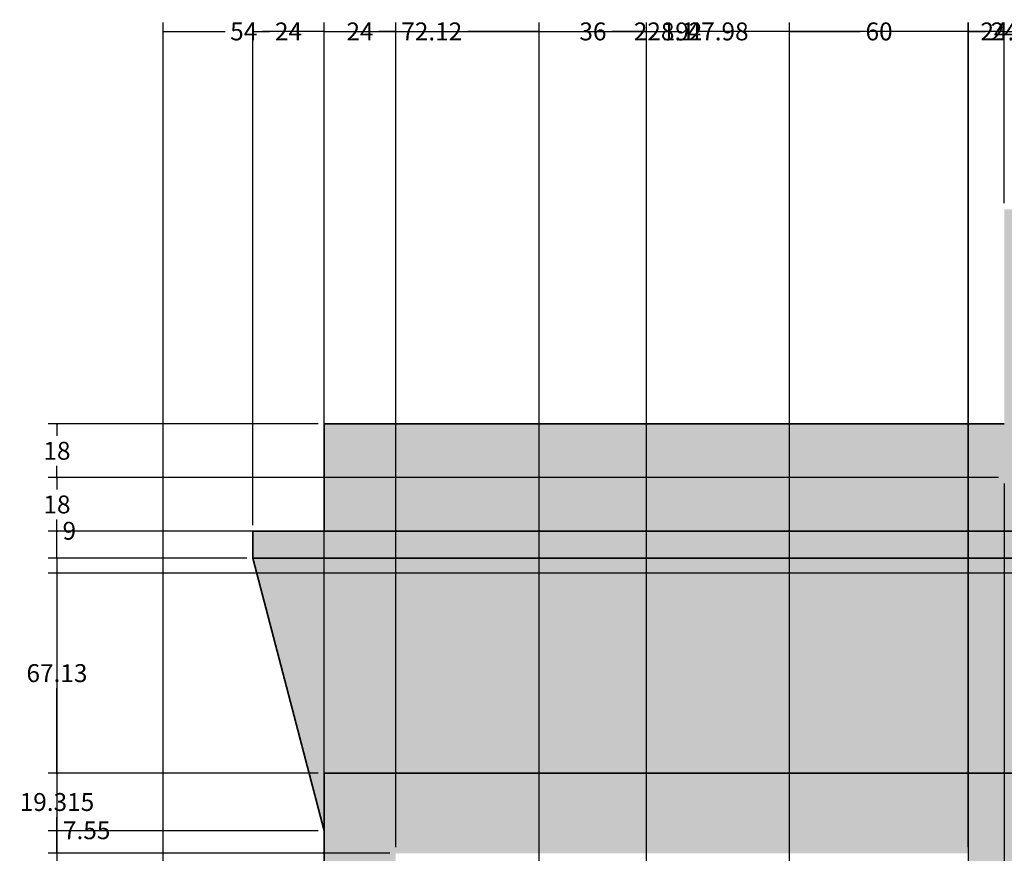
# Model space of a CAD drawing. Units: inches. Extents: x 860 to 1491, y 583 to 1370.
# Tile 7 of 8: x 860 to 1190, y 1091 to 1370. Entities that reach past the tile are written whole.
import ezdxf

# ---------------------------------------------------------------- set-up
doc = ezdxf.new("R2010")
doc.units = ezdxf.units.IN
doc.header["$MEASUREMENT"] = 0
doc.layers.get('0').update_dxf_attribs({"color": 250})
for name, color, linetype, lineweight in [('A-ANNO-DIMS', 2, 'Continuous', 18), ('A-ELEV', 7, 'Continuous', 35), ('A-ELEV-PATT', 9, 'Continuous', 13)]:
    doc.layers.add(name, color=color, linetype=linetype, lineweight=lineweight)
doc.styles.get("Standard").update_dxf_attribs({"font": 'arial.ttf'})
doc.dimstyles.get("Standard").update_dxf_attribs({"dimtxt": 6, "dimasz": 0.18, "dimexe": 3, "dimexo": 2, "dimgap": 2, "dimtad": 0, "dimtih": 1, "dimtoh": 1, "dimdec": 0, "dimzin": 0, "dimdsep": 46, "dimlunit": 3, "dimtxsty": 'Standard', "dimblk2": 'CLOSEDBLANK', "dimsah": 1, "dimcen": 2, "dimadec": 0, "dimazin": 0, "dimtfac": 1, "dimtdec": 0, "dimtofl": 0, "dimtmove": 0, "dimatfit": 3, "dimfxl": 1, "dimtolj": 1, "dimtzin": 0, "dimarcsym": 0})

# ---------------------------------------------------------------- blocks, each defined once
blk = doc.blocks.new('_ClosedBlank')
at = {"color": 0, "linetype": 'ByBlock', "lineweight": -2}
for p, q in [((-1, 0.17), (0, 0)), ((-1, 0.17), (-1, -0.17)), ((0, 0), (-1, -0.17))]:
    blk.add_line(p, q, dxfattribs=at)
blk = doc.blocks.new('*D2')
at = {"layer": 'A-ANNO-DIMS', "color": 0, "lineweight": -2, "transparency": 16777216}
for p, q in [((1442.44, 1328.76), (1442.44, 584.11)), ((908.34, 740.76), (908.34, 584.11)), ((908.52, 587.11), (1163.85, 587.11)), ((1442.26, 587.11), (1186.93, 587.11))]:
    blk.add_line(p, q, dxfattribs=at)
at = {"layer": 'A-ANNO-DIMS', "color": 0, "transparency": 16777216}
blk.add_solid([(908.52, 587.14), (908.52, 587.08), (908.34, 587.11)], dxfattribs=at)
at = {"layer": 'Defpoints', "color": 0, "transparency": 16777216}
for p in [(1442.44, 1330.76), (908.34, 742.76), (1442.44, 587.11)]:
    blk.add_point(p, dxfattribs=at)
at = {"layer": 'A-ANNO-DIMS', "color": 0, "lineweight": -2, "transparency": 16777216, "xscale": 0.18, "yscale": 0.18, "zscale": 0.18}
blk.add_blockref('_ClosedBlank', (1442.44, 587.11), dxfattribs=at)
at = {"layer": 'A-ANNO-DIMS', "color": 0, "transparency": 16777216, "insert": (1175.39, 587.11), "char_height": 6, "attachment_point": 5}
blk.add_mtext('\\A1;534.1', dxfattribs=at)
blk = doc.blocks.new('*D5')
at = {"layer": 'A-ANNO-DIMS', "color": 0, "lineweight": -2, "transparency": 16777216}
for p, q in [((936.34, 1189.76), (869.69, 1189.76)), ((872.69, 1189.58), (872.69, 1049.32)), ((872.69, 898.94), (872.69, 1039.19)), ((960.34, 898.76), (869.69, 898.76))]:
    blk.add_line(p, q, dxfattribs=at)
at = {"layer": 'A-ANNO-DIMS', "color": 0, "transparency": 16777216}
blk.add_solid([(872.66, 898.94), (872.72, 898.94), (872.69, 898.76)], dxfattribs=at)
at = {"layer": 'Defpoints', "color": 0, "transparency": 16777216}
for p in [(872.69, 1189.76), (938.34, 1189.76), (962.34, 898.76)]:
    blk.add_point(p, dxfattribs=at)
at = {"layer": 'A-ANNO-DIMS', "color": 0, "lineweight": -2, "transparency": 16777216, "xscale": 0.18, "yscale": 0.18, "zscale": 0.18, "rotation": 90}
blk.add_blockref('_ClosedBlank', (872.69, 1189.76), dxfattribs=at)
at = {"layer": 'A-ANNO-DIMS', "color": 0, "transparency": 16777216, "insert": (872.69, 1044.26), "char_height": 6, "attachment_point": 5}
blk.add_mtext('\\A1;291', dxfattribs=at)
blk = doc.blocks.new('*D20')
at = {"layer": 'A-ANNO-DIMS', "color": 0, "lineweight": -2, "transparency": 16777216}
for p, q in [((908.34, 744.76), (908.34, 1369.41)), ((962.34, 732.76), (962.34, 1369.41)), ((908.52, 1366.41), (929.06, 1366.41)), ((962.16, 1366.41), (941.63, 1366.41))]:
    blk.add_line(p, q, dxfattribs=at)
at = {"layer": 'A-ANNO-DIMS', "color": 0, "transparency": 16777216}
blk.add_solid([(908.52, 1366.44), (908.52, 1366.38), (908.34, 1366.41)], dxfattribs=at)
at = {"layer": 'Defpoints', "color": 0, "transparency": 16777216}
for p in [(962.34, 1366.41), (908.34, 742.76), (962.34, 730.76)]:
    blk.add_point(p, dxfattribs=at)
at = {"layer": 'A-ANNO-DIMS', "color": 0, "lineweight": -2, "transparency": 16777216, "xscale": 0.18, "yscale": 0.18, "zscale": 0.18}
blk.add_blockref('_ClosedBlank', (962.34, 1366.41), dxfattribs=at)
at = {"layer": 'A-ANNO-DIMS', "color": 0, "transparency": 16777216, "insert": (935.34, 1366.41), "char_height": 6, "attachment_point": 5}
blk.add_mtext('\\A1;54', dxfattribs=at)
blk = doc.blocks.new('*D21')
at = {"layer": 'A-ANNO-DIMS', "color": 0, "lineweight": -2, "transparency": 16777216}
for p, q in [((962.34, 732.76), (962.34, 1369.41)), ((1034.46, 828.76), (1034.46, 1369.41)), ((962.52, 1366.41), (986.33, 1366.41)), ((1034.28, 1366.41), (1010.47, 1366.41))]:
    blk.add_line(p, q, dxfattribs=at)
at = {"layer": 'A-ANNO-DIMS', "color": 0, "transparency": 16777216}
blk.add_solid([(962.52, 1366.44), (962.52, 1366.38), (962.34, 1366.41)], dxfattribs=at)
at = {"layer": 'Defpoints', "color": 0, "transparency": 16777216}
for p in [(1034.46, 1366.41), (1034.46, 826.76), (962.34, 730.76)]:
    blk.add_point(p, dxfattribs=at)
at = {"layer": 'A-ANNO-DIMS', "color": 0, "lineweight": -2, "transparency": 16777216, "xscale": 0.18, "yscale": 0.18, "zscale": 0.18}
blk.add_blockref('_ClosedBlank', (1034.46, 1366.41), dxfattribs=at)
at = {"layer": 'A-ANNO-DIMS', "color": 0, "transparency": 16777216, "insert": (998.4, 1366.41), "char_height": 6, "attachment_point": 5}
blk.add_mtext('\\A1;72.12', dxfattribs=at)
blk = doc.blocks.new('*D22')
at = {"layer": 'A-ANNO-DIMS', "color": 0, "lineweight": -2, "transparency": 16777216}
for p, q in [((1034.46, 828.76), (1034.46, 1369.41)), ((1070.46, 828.76), (1070.46, 1369.41)), ((1034.64, 1366.41), (1046.17, 1366.41)), ((1070.28, 1366.41), (1058.75, 1366.41))]:
    blk.add_line(p, q, dxfattribs=at)
at = {"layer": 'A-ANNO-DIMS', "color": 0, "transparency": 16777216}
blk.add_solid([(1034.64, 1366.44), (1034.64, 1366.38), (1034.46, 1366.41)], dxfattribs=at)
at = {"layer": 'Defpoints', "color": 0, "transparency": 16777216}
for p in [(1070.46, 1366.41), (1034.46, 826.76), (1070.46, 826.76)]:
    blk.add_point(p, dxfattribs=at)
at = {"layer": 'A-ANNO-DIMS', "color": 0, "lineweight": -2, "transparency": 16777216, "xscale": 0.18, "yscale": 0.18, "zscale": 0.18}
blk.add_blockref('_ClosedBlank', (1070.46, 1366.41), dxfattribs=at)
at = {"layer": 'A-ANNO-DIMS', "color": 0, "transparency": 16777216, "insert": (1052.46, 1366.41), "char_height": 6, "attachment_point": 5}
blk.add_mtext('\\A1;36', dxfattribs=at)
blk = doc.blocks.new('*D23')
at = {"layer": 'A-ANNO-DIMS', "color": 0, "lineweight": -2, "transparency": 16777216}
for p, q in [((1070.46, 828.76), (1070.46, 1369.41)), ((1118.44, 840.76), (1118.44, 1369.41)), ((1070.64, 1366.41), (1082.2, 1366.41)), ((1118.26, 1366.41), (1106.7, 1366.41))]:
    blk.add_line(p, q, dxfattribs=at)
at = {"layer": 'A-ANNO-DIMS', "color": 0, "transparency": 16777216}
blk.add_solid([(1070.64, 1366.44), (1070.64, 1366.38), (1070.46, 1366.41)], dxfattribs=at)
at = {"layer": 'Defpoints', "color": 0, "transparency": 16777216}
for p in [(1118.44, 1366.41), (1118.44, 838.76), (1070.46, 826.76)]:
    blk.add_point(p, dxfattribs=at)
at = {"layer": 'A-ANNO-DIMS', "color": 0, "lineweight": -2, "transparency": 16777216, "xscale": 0.18, "yscale": 0.18, "zscale": 0.18}
blk.add_blockref('_ClosedBlank', (1118.44, 1366.41), dxfattribs=at)
at = {"layer": 'A-ANNO-DIMS', "color": 0, "transparency": 16777216, "insert": (1094.45, 1366.41), "char_height": 6, "attachment_point": 5}
blk.add_mtext('\\A1;47.98', dxfattribs=at)
blk = doc.blocks.new('*D24')
at = {"layer": 'A-ANNO-DIMS', "color": 0, "lineweight": -2, "transparency": 16777216}
for p, q in [((1118.44, 840.76), (1118.44, 1369.41)), ((1178.44, 840.76), (1178.44, 1369.41)), ((1118.62, 1366.41), (1142.14, 1366.41)), ((1178.26, 1366.41), (1154.74, 1366.41))]:
    blk.add_line(p, q, dxfattribs=at)
at = {"layer": 'A-ANNO-DIMS', "color": 0, "transparency": 16777216}
blk.add_solid([(1118.62, 1366.44), (1118.62, 1366.38), (1118.44, 1366.41)], dxfattribs=at)
at = {"layer": 'Defpoints', "color": 0, "transparency": 16777216}
for p in [(1178.44, 1366.41), (1118.44, 838.76), (1178.44, 838.76)]:
    blk.add_point(p, dxfattribs=at)
at = {"layer": 'A-ANNO-DIMS', "color": 0, "lineweight": -2, "transparency": 16777216, "xscale": 0.18, "yscale": 0.18, "zscale": 0.18}
blk.add_blockref('_ClosedBlank', (1178.44, 1366.41), dxfattribs=at)
at = {"layer": 'A-ANNO-DIMS', "color": 0, "transparency": 16777216, "insert": (1148.44, 1366.41), "char_height": 6, "attachment_point": 5}
blk.add_mtext('\\A1;60', dxfattribs=at)
blk = doc.blocks.new('*D25')
at = {"layer": 'A-ANNO-DIMS', "color": 0, "lineweight": -2, "transparency": 16777216}
for p, q in [((1178.44, 840.76), (1178.44, 1369.41)), ((1202.44, 744.76), (1202.44, 1369.41)), ((1178.62, 1366.41), (1184.1, 1366.41)), ((1202.26, 1366.41), (1196.78, 1366.41))]:
    blk.add_line(p, q, dxfattribs=at)
at = {"layer": 'A-ANNO-DIMS', "color": 0, "transparency": 16777216}
blk.add_solid([(1178.62, 1366.44), (1178.62, 1366.38), (1178.44, 1366.41)], dxfattribs=at)
at = {"layer": 'Defpoints', "color": 0, "transparency": 16777216}
for p in [(1202.44, 1366.41), (1178.44, 838.76), (1202.44, 742.76)]:
    blk.add_point(p, dxfattribs=at)
at = {"layer": 'A-ANNO-DIMS', "color": 0, "lineweight": -2, "transparency": 16777216, "xscale": 0.18, "yscale": 0.18, "zscale": 0.18}
blk.add_blockref('_ClosedBlank', (1202.44, 1366.41), dxfattribs=at)
at = {"layer": 'A-ANNO-DIMS', "color": 0, "transparency": 16777216, "insert": (1190.44, 1366.41), "char_height": 6, "attachment_point": 5}
blk.add_mtext('\\A1;24', dxfattribs=at)
blk = doc.blocks.new('*D44')
at = {"layer": 'A-ANNO-DIMS', "color": 0, "lineweight": -2, "transparency": 16777216}
for p, q in [((984.340309, 1090.755507), (869.690309, 1090.755507)), ((872.690309, 1090.935507), (872.690309, 1091.115507)), ((996.340309, 1078.755507), (869.690309, 1078.755507)), ((872.690309, 1078.575507), (872.690309, 1078.395507))]:
    blk.add_line(p, q, dxfattribs=at)
at = {"layer": 'A-ANNO-DIMS', "color": 0, "transparency": 16777216}
blk.add_solid([(872.660309, 1078.575507), (872.720309, 1078.575507), (872.690309, 1078.755507)], dxfattribs=at)
at = {"layer": 'Defpoints', "color": 0, "transparency": 16777216}
for p in [(872.690309, 1090.755507), (986.340309, 1090.755507), (998.340309, 1078.755507)]:
    blk.add_point(p, dxfattribs=at)
at = {"layer": 'A-ANNO-DIMS', "color": 0, "lineweight": -2, "transparency": 16777216, "xscale": 0.18, "yscale": 0.18, "zscale": 0.18, "rotation": 270}
blk.add_blockref('_ClosedBlank', (872.690309, 1090.755507), dxfattribs=at)
at = {"layer": 'A-ANNO-DIMS', "color": 0, "transparency": 16777216, "insert": (872.690309, 1084.755507), "char_height": 6, "attachment_point": 5}
blk.add_mtext('\\A1;12', dxfattribs=at)
blk = doc.blocks.new('*D45')
at = {"layer": 'A-ANNO-DIMS', "color": 0, "lineweight": -2, "transparency": 16777216}
for p, q in [((960.34, 1098.31), (869.69, 1098.31)), ((872.69, 1098.31), (872.69, 1098.49)), ((872.69, 1098.49), (872.87, 1098.49)), ((872.69, 1090.94), (872.69, 1098.13)), ((984.34, 1090.76), (869.69, 1090.76))]:
    blk.add_line(p, q, dxfattribs=at)
at = {"layer": 'A-ANNO-DIMS', "color": 0, "transparency": 16777216}
blk.add_solid([(872.66, 1090.94), (872.72, 1090.94), (872.69, 1090.76)], dxfattribs=at)
at = {"layer": 'Defpoints', "color": 0, "transparency": 16777216}
for p in [(872.69, 1098.31), (962.34, 1098.31), (986.34, 1090.76)]:
    blk.add_point(p, dxfattribs=at)
at = {"layer": 'A-ANNO-DIMS', "color": 0, "lineweight": -2, "transparency": 16777216, "xscale": 0.18, "yscale": 0.18, "zscale": 0.18, "rotation": 90}
blk.add_blockref('_ClosedBlank', (872.69, 1098.31), dxfattribs=at)
at = {"layer": 'A-ANNO-DIMS', "color": 0, "transparency": 16777216, "insert": (882.66, 1098.49), "char_height": 6, "attachment_point": 5}
blk.add_mtext('\\A1;7.55', dxfattribs=at)
blk = doc.blocks.new('*D46')
at = {"layer": 'A-ANNO-DIMS', "color": 0, "lineweight": -2, "transparency": 16777216}
for p, q in [((960.34, 1117.62), (869.69, 1117.62)), ((872.69, 1117.44), (872.69, 1113.03)), ((872.69, 1098.49), (872.69, 1102.9)), ((960.34, 1098.31), (869.69, 1098.31))]:
    blk.add_line(p, q, dxfattribs=at)
at = {"layer": 'A-ANNO-DIMS', "color": 0, "transparency": 16777216}
blk.add_solid([(872.66, 1098.49), (872.72, 1098.49), (872.69, 1098.31)], dxfattribs=at)
at = {"layer": 'Defpoints', "color": 0, "transparency": 16777216}
for p in [(872.69, 1117.62), (962.34, 1117.62), (962.34, 1098.31)]:
    blk.add_point(p, dxfattribs=at)
at = {"layer": 'A-ANNO-DIMS', "color": 0, "lineweight": -2, "transparency": 16777216, "xscale": 0.18, "yscale": 0.18, "zscale": 0.18, "rotation": 90}
blk.add_blockref('_ClosedBlank', (872.69, 1117.62), dxfattribs=at)
at = {"layer": 'A-ANNO-DIMS', "color": 0, "transparency": 16777216, "insert": (872.69, 1107.96), "char_height": 6, "attachment_point": 5}
blk.add_mtext('\\A1;19.315', dxfattribs=at)
blk = doc.blocks.new('*D47')
at = {"layer": 'A-ANNO-DIMS', "color": 0, "lineweight": -2, "transparency": 16777216}
for p, q in [((1200.44, 1184.76), (869.69, 1184.76)), ((872.69, 1184.58), (872.69, 1156.25)), ((872.69, 1117.8), (872.69, 1146.12)), ((960.34, 1117.62), (869.69, 1117.62))]:
    blk.add_line(p, q, dxfattribs=at)
at = {"layer": 'A-ANNO-DIMS', "color": 0, "transparency": 16777216}
blk.add_solid([(872.66, 1117.8), (872.72, 1117.8), (872.69, 1117.62)], dxfattribs=at)
at = {"layer": 'Defpoints', "color": 0, "transparency": 16777216}
for p in [(872.69, 1184.76), (1202.44, 1184.76), (962.34, 1117.62)]:
    blk.add_point(p, dxfattribs=at)
at = {"layer": 'A-ANNO-DIMS', "color": 0, "lineweight": -2, "transparency": 16777216, "xscale": 0.18, "yscale": 0.18, "zscale": 0.18, "rotation": 90}
blk.add_blockref('_ClosedBlank', (872.69, 1184.76), dxfattribs=at)
at = {"layer": 'A-ANNO-DIMS', "color": 0, "transparency": 16777216, "insert": (872.69, 1151.19), "char_height": 6, "attachment_point": 5}
blk.add_mtext('\\A1;67.13', dxfattribs=at)
blk = doc.blocks.new('*D55')
at = {"layer": 'A-ANNO-DIMS', "color": 0, "lineweight": -2, "transparency": 16777216}
for p, q in [((962.34, 1119.62), (962.34, 1369.41)), ((986.34, 1092.76), (986.34, 1369.41)), ((962.52, 1366.41), (968, 1366.41)), ((986.16, 1366.41), (980.68, 1366.41))]:
    blk.add_line(p, q, dxfattribs=at)
at = {"layer": 'A-ANNO-DIMS', "color": 0, "transparency": 16777216}
blk.add_solid([(962.52, 1366.44), (962.52, 1366.38), (962.34, 1366.41)], dxfattribs=at)
at = {"layer": 'Defpoints', "color": 0, "transparency": 16777216}
for p in [(986.34, 1366.41), (962.34, 1117.62), (986.34, 1090.76)]:
    blk.add_point(p, dxfattribs=at)
at = {"layer": 'A-ANNO-DIMS', "color": 0, "lineweight": -2, "transparency": 16777216, "xscale": 0.18, "yscale": 0.18, "zscale": 0.18}
blk.add_blockref('_ClosedBlank', (986.34, 1366.41), dxfattribs=at)
at = {"layer": 'A-ANNO-DIMS', "color": 0, "transparency": 16777216, "insert": (974.34, 1366.41), "char_height": 6, "attachment_point": 5}
blk.add_mtext('\\A1;24', dxfattribs=at)
blk = doc.blocks.new('*D56')
at = {"layer": 'A-ANNO-DIMS', "color": 0, "lineweight": -2, "transparency": 16777216}
for p, q in [((986.34, 1092.76), (986.34, 1369.41)), ((1178.34, 1092.76), (1178.34, 1369.41)), ((986.52, 1366.41), (1074.03, 1366.41)), ((1178.16, 1366.41), (1090.66, 1366.41))]:
    blk.add_line(p, q, dxfattribs=at)
at = {"layer": 'A-ANNO-DIMS', "color": 0, "transparency": 16777216}
blk.add_solid([(986.52, 1366.44), (986.52, 1366.38), (986.34, 1366.41)], dxfattribs=at)
at = {"layer": 'Defpoints', "color": 0, "transparency": 16777216}
for p in [(1178.34, 1366.41), (986.34, 1090.76), (1178.34, 1090.76)]:
    blk.add_point(p, dxfattribs=at)
at = {"layer": 'A-ANNO-DIMS', "color": 0, "lineweight": -2, "transparency": 16777216, "xscale": 0.18, "yscale": 0.18, "zscale": 0.18}
blk.add_blockref('_ClosedBlank', (1178.34, 1366.41), dxfattribs=at)
at = {"layer": 'A-ANNO-DIMS', "color": 0, "transparency": 16777216, "insert": (1082.34, 1366.41), "char_height": 6, "attachment_point": 5}
blk.add_mtext('\\A1;192', dxfattribs=at)
blk = doc.blocks.new('*D57')
at = {"layer": 'A-ANNO-DIMS', "color": 0, "lineweight": -2, "transparency": 16777216}
for p, q in [((1178.34, 1092.76), (1178.34, 1369.41)), ((1202.44, 1186.76), (1202.44, 1369.41)), ((1178.52, 1366.41), (1181.13, 1366.41)), ((1202.26, 1366.41), (1199.65, 1366.41))]:
    blk.add_line(p, q, dxfattribs=at)
at = {"layer": 'A-ANNO-DIMS', "color": 0, "transparency": 16777216}
blk.add_solid([(1178.52, 1366.44), (1178.52, 1366.38), (1178.34, 1366.41)], dxfattribs=at)
at = {"layer": 'Defpoints', "color": 0, "transparency": 16777216}
for p in [(1202.44, 1366.41), (1202.44, 1184.76), (1178.34, 1090.76)]:
    blk.add_point(p, dxfattribs=at)
at = {"layer": 'A-ANNO-DIMS', "color": 0, "lineweight": -2, "transparency": 16777216, "xscale": 0.18, "yscale": 0.18, "zscale": 0.18}
blk.add_blockref('_ClosedBlank', (1202.44, 1366.41), dxfattribs=at)
at = {"layer": 'A-ANNO-DIMS', "color": 0, "transparency": 16777216, "insert": (1190.39, 1366.41), "char_height": 6, "attachment_point": 5}
blk.add_mtext('\\A1;24.1', dxfattribs=at)
blk = doc.blocks.new('*D71')
at = {"layer": 'A-ANNO-DIMS', "color": 0, "lineweight": -2, "transparency": 16777216}
for p, q in [((938.34, 1200.76), (938.34, 1369.41)), ((962.34, 1236.76), (962.34, 1369.41)), ((938.52, 1366.41), (944, 1366.41)), ((962.16, 1366.41), (956.68, 1366.41))]:
    blk.add_line(p, q, dxfattribs=at)
at = {"layer": 'A-ANNO-DIMS', "color": 0, "transparency": 16777216}
blk.add_solid([(938.52, 1366.44), (938.52, 1366.38), (938.34, 1366.41)], dxfattribs=at)
at = {"layer": 'Defpoints', "color": 0, "transparency": 16777216}
for p in [(962.34, 1366.41), (962.34, 1234.76), (938.34, 1198.76)]:
    blk.add_point(p, dxfattribs=at)
at = {"layer": 'A-ANNO-DIMS', "color": 0, "lineweight": -2, "transparency": 16777216, "xscale": 0.18, "yscale": 0.18, "zscale": 0.18}
blk.add_blockref('_ClosedBlank', (962.34, 1366.41), dxfattribs=at)
at = {"layer": 'A-ANNO-DIMS', "color": 0, "transparency": 16777216, "insert": (950.34, 1366.41), "char_height": 6, "attachment_point": 5}
blk.add_mtext('\\A1;24', dxfattribs=at)
blk = doc.blocks.new('*D72')
at = {"layer": 'A-ANNO-DIMS', "color": 0, "lineweight": -2, "transparency": 16777216}
for p, q in [((962.34, 1236.76), (962.34, 1369.41)), ((1190.44, 1308.76), (1190.44, 1369.41)), ((962.52, 1366.41), (1064.79, 1366.41)), ((1190.26, 1366.41), (1087.99, 1366.41))]:
    blk.add_line(p, q, dxfattribs=at)
at = {"layer": 'A-ANNO-DIMS', "color": 0, "transparency": 16777216}
blk.add_solid([(962.52, 1366.44), (962.52, 1366.38), (962.34, 1366.41)], dxfattribs=at)
at = {"layer": 'Defpoints', "color": 0, "transparency": 16777216}
for p in [(1190.44, 1366.41), (1190.44, 1306.76), (962.34, 1234.76)]:
    blk.add_point(p, dxfattribs=at)
at = {"layer": 'A-ANNO-DIMS', "color": 0, "lineweight": -2, "transparency": 16777216, "xscale": 0.18, "yscale": 0.18, "zscale": 0.18}
blk.add_blockref('_ClosedBlank', (1190.44, 1366.41), dxfattribs=at)
at = {"layer": 'A-ANNO-DIMS', "color": 0, "transparency": 16777216, "insert": (1076.39, 1366.41), "char_height": 6, "attachment_point": 5}
blk.add_mtext('\\A1;228.1', dxfattribs=at)
blk = doc.blocks.new('*D73')
at = {"layer": 'A-ANNO-DIMS', "color": 0, "lineweight": -2, "transparency": 16777216}
for p, q in [((1190.44, 1308.76), (1190.44, 1369.41)), ((1358.44, 1308.76), (1358.44, 1369.41)), ((1190.62, 1366.41), (1266.09, 1366.41)), ((1358.26, 1366.41), (1282.79, 1366.41))]:
    blk.add_line(p, q, dxfattribs=at)
at = {"layer": 'A-ANNO-DIMS', "color": 0, "transparency": 16777216}
blk.add_solid([(1190.62, 1366.44), (1190.62, 1366.38), (1190.44, 1366.41)], dxfattribs=at)
at = {"layer": 'Defpoints', "color": 0, "transparency": 16777216}
for p in [(1358.44, 1366.41), (1190.44, 1306.76), (1358.44, 1306.76)]:
    blk.add_point(p, dxfattribs=at)
at = {"layer": 'A-ANNO-DIMS', "color": 0, "lineweight": -2, "transparency": 16777216, "xscale": 0.18, "yscale": 0.18, "zscale": 0.18}
blk.add_blockref('_ClosedBlank', (1358.44, 1366.41), dxfattribs=at)
at = {"layer": 'A-ANNO-DIMS', "color": 0, "transparency": 16777216, "insert": (1274.44, 1366.41), "char_height": 6, "attachment_point": 5}
blk.add_mtext('\\A1;168', dxfattribs=at)
blk = doc.blocks.new('*D76')
at = {"layer": 'A-ANNO-DIMS', "color": 0, "lineweight": -2, "transparency": 16777216}
for p, q in [((1202.440309, 1277.755507), (1202.440309, 584.105507)), ((1190.440309, 1214.755507), (1190.440309, 584.105507)), ((1190.260309, 587.105507), (1190.080309, 587.105507)), ((1202.620309, 587.105507), (1202.800309, 587.105507))]:
    blk.add_line(p, q, dxfattribs=at)
at = {"layer": 'A-ANNO-DIMS', "color": 0, "transparency": 16777216}
blk.add_solid([(1190.260309, 587.135507), (1190.260309, 587.075507), (1190.440309, 587.105507)], dxfattribs=at)
at = {"layer": 'Defpoints', "color": 0, "transparency": 16777216}
for p in [(1202.440309, 1279.755507), (1190.440309, 1216.755507), (1202.440309, 587.105507)]:
    blk.add_point(p, dxfattribs=at)
at = {"layer": 'A-ANNO-DIMS', "color": 0, "lineweight": -2, "transparency": 16777216, "xscale": 0.18, "yscale": 0.18, "zscale": 0.18, "rotation": 180}
blk.add_blockref('_ClosedBlank', (1202.440309, 587.105507), dxfattribs=at)
at = {"layer": 'A-ANNO-DIMS', "color": 0, "transparency": 16777216, "insert": (1196.440309, 587.105507), "char_height": 6, "attachment_point": 5}
blk.add_mtext('\\A1;12', dxfattribs=at)
blk = doc.blocks.new('*D79')
at = {"layer": 'A-ANNO-DIMS', "color": 0, "lineweight": -2, "transparency": 16777216}
for p, q in [((872.69, 1198.76), (872.69, 1198.94)), ((872.69, 1198.94), (872.87, 1198.94)), ((936.34, 1198.76), (869.69, 1198.76)), ((872.69, 1189.94), (872.69, 1198.58)), ((936.34, 1189.76), (869.69, 1189.76))]:
    blk.add_line(p, q, dxfattribs=at)
at = {"layer": 'A-ANNO-DIMS', "color": 0, "transparency": 16777216}
blk.add_solid([(872.66, 1189.94), (872.72, 1189.94), (872.69, 1189.76)], dxfattribs=at)
at = {"layer": 'Defpoints', "color": 0, "transparency": 16777216}
for p in [(872.69, 1198.76), (938.34, 1198.76), (938.34, 1189.76)]:
    blk.add_point(p, dxfattribs=at)
at = {"layer": 'A-ANNO-DIMS', "color": 0, "lineweight": -2, "transparency": 16777216, "xscale": 0.18, "yscale": 0.18, "zscale": 0.18, "rotation": 90}
blk.add_blockref('_ClosedBlank', (872.69, 1198.76), dxfattribs=at)
at = {"layer": 'A-ANNO-DIMS', "color": 0, "transparency": 16777216, "insert": (876.84, 1198.94), "char_height": 6, "attachment_point": 5}
blk.add_mtext('\\A1;9', dxfattribs=at)
blk = doc.blocks.new('*D80')
at = {"layer": 'A-ANNO-DIMS', "color": 0, "lineweight": -2, "transparency": 16777216}
for p, q in [((1188.44, 1216.76), (869.69, 1216.76)), ((872.69, 1216.58), (872.69, 1212.82)), ((872.69, 1198.94), (872.69, 1202.69)), ((960.34, 1198.76), (869.69, 1198.76))]:
    blk.add_line(p, q, dxfattribs=at)
at = {"layer": 'A-ANNO-DIMS', "color": 0, "transparency": 16777216}
blk.add_solid([(872.66, 1198.94), (872.72, 1198.94), (872.69, 1198.76)], dxfattribs=at)
at = {"layer": 'Defpoints', "color": 0, "transparency": 16777216}
for p in [(872.69, 1216.76), (1190.44, 1216.76), (962.34, 1198.76)]:
    blk.add_point(p, dxfattribs=at)
at = {"layer": 'A-ANNO-DIMS', "color": 0, "lineweight": -2, "transparency": 16777216, "xscale": 0.18, "yscale": 0.18, "zscale": 0.18, "rotation": 90}
blk.add_blockref('_ClosedBlank', (872.69, 1216.76), dxfattribs=at)
at = {"layer": 'A-ANNO-DIMS', "color": 0, "transparency": 16777216, "insert": (872.69, 1207.76), "char_height": 6, "attachment_point": 5}
blk.add_mtext('\\A1;18', dxfattribs=at)
blk = doc.blocks.new('*D81')
at = {"layer": 'A-ANNO-DIMS', "color": 0, "lineweight": -2, "transparency": 16777216}
for p, q in [((960.34, 1234.76), (869.69, 1234.76)), ((872.69, 1234.58), (872.69, 1230.82)), ((872.69, 1216.94), (872.69, 1220.69)), ((1188.44, 1216.76), (869.69, 1216.76))]:
    blk.add_line(p, q, dxfattribs=at)
at = {"layer": 'A-ANNO-DIMS', "color": 0, "transparency": 16777216}
blk.add_solid([(872.66, 1216.94), (872.72, 1216.94), (872.69, 1216.76)], dxfattribs=at)
at = {"layer": 'Defpoints', "color": 0, "transparency": 16777216}
for p in [(872.69, 1234.76), (962.34, 1234.76), (1190.44, 1216.76)]:
    blk.add_point(p, dxfattribs=at)
at = {"layer": 'A-ANNO-DIMS', "color": 0, "lineweight": -2, "transparency": 16777216, "xscale": 0.18, "yscale": 0.18, "zscale": 0.18, "rotation": 90}
blk.add_blockref('_ClosedBlank', (872.69, 1234.76), dxfattribs=at)
at = {"layer": 'A-ANNO-DIMS', "color": 0, "transparency": 16777216, "insert": (872.69, 1225.76), "char_height": 6, "attachment_point": 5}
blk.add_mtext('\\A1;18', dxfattribs=at)

msp = doc.modelspace()

# ---------------------------------------------------------------- hatches: boundary and pattern name
at = {"layer": 'A-ELEV-PATT'}
h = msp.add_hatch(color=256, dxfattribs=at)
h.dxf.hatch_style = 1
h.paths.add_polyline_path([(1442.4403, 1330.7555), (1370.4403, 1330.7555), (1370.4403, 622.7555), (1442.4403, 622.7555)])
h.paths.add_polyline_path([(1358.4403, 1306.7555), (1190.4403, 1306.7555), (1190.4403, 1288.7555), (1358.4403, 1288.7555)])
h.paths.add_polyline_path([(1190.4403, 1234.7555), (962.3403, 1234.7555), (962.3403, 1198.7555), (1202.4403, 1198.7555), (1202.4403, 1216.7555), (1190.4403, 1216.7555)])
h.paths.add_polyline_path([(1202.4403, 1117.6207), (962.3403, 1117.6207), (962.3403, 982.7555), (986.3403, 982.7555), (986.3403, 1090.7555), (1178.3403, 1090.7555), (1178.3403, 982.7555), (1202.4403, 982.7555)])
h.paths.add_polyline_path([(1319.4403, 1184.7555), (1202.4403, 1184.7555), (1202.4403, 982.7555), (1211.4403, 982.7555), (1211.4403, 946.7555), (1220.4403, 946.7555), (1220.4403, 934.7555), (1319.4403, 934.7555)])
h.paths.add_polyline_path([(1271.4403, 1160.7555), (1307.4403, 1160.7555), (1307.4403, 944.7555), (1271.4403, 944.7555)], flags=16)
h.paths.add_polyline_path([(1275.4403, 1156.7555), (1303.4403, 1156.7555), (1303.4403, 948.7555), (1275.4403, 948.7555)], flags=0)
h.paths.add_polyline_path([(1202.4403, 898.7555), (962.3403, 898.7555), (962.3403, 730.7555), (1034.4585, 730.7555), (1034.4585, 826.7555), (1070.4585, 826.7555), (1070.4585, 730.7555), (1118.4403, 730.7555), (1118.4403, 838.7555), (1178.4403, 838.7555), (1178.4403, 730.7555), (1202.4403, 730.7555)])
h.paths.add_polyline_path([(1220.4403, 946.7555), (1211.4403, 946.7555), (938.3403, 946.7555), (926.3403, 946.7555), (926.3403, 910.7555), (962.3403, 910.7555), (1220.4403, 910.7555)])
h.paths.add_polyline_path([(950.3403, 730.7555), (950.3403, 734.7555), (938.3403, 742.7555), (938.3403, 730.7555), (938.3403, 622.7555), (950.3403, 622.7555)])
h = msp.add_hatch(color=256, dxfattribs=at)
h.dxf.hatch_style = 1
h.paths.add_polyline_path([(1202.4403, 1184.7555), (1319.4403, 1184.7555), (1328.4403, 1189.7555), (938.3403, 1189.7555), (962.3403, 1098.3061), (962.3403, 1117.6207), (1202.4403, 1117.6207)])
h.paths.add_polyline_path([(1202.4403, 1198.7555), (938.3403, 1198.7555), (938.3403, 1189.7555), (1202.4403, 1189.7555)])
h.paths.add_polyline_path([(1328.4403, 1198.7555), (1202.4403, 1198.7555), (1202.4403, 1189.7555), (1328.4403, 1189.7555)])
h.paths.add_polyline_path([(1328.4403, 1189.7555), (1319.4403, 1184.7555), (1319.4403, 934.7555), (1328.4403, 934.7555)])
h.paths.add_polyline_path([(1328.4403, 934.7555), (1319.4403, 934.7555), (1220.4403, 934.7555), (1220.4403, 922.7555), (1328.4403, 922.7555)])
h.paths.add_polyline_path([(1202.4403, 1279.7555), (1190.4403, 1279.7555), (1190.4403, 1216.7555), (1202.4403, 1216.7555)])
h.paths.add_polyline_path([(1358.4403, 1288.7555), (1190.4403, 1288.7555), (1190.4403, 1279.7555), (1352.4403, 1279.7555)])
h.paths.add_polyline_path([(1370.4403, 1330.7555), (1352.4403, 1318.7555), (1352.4403, 1306.7555), (1358.4403, 1306.7555), (1358.4403, 1288.7555), (1352.4403, 1279.7555), (1352.4403, 730.7555), (1370.4403, 730.7555)])

# ---------------------------------------------------------------- linework, layer by layer
at = {"layer": 'A-ELEV'}
for p, q in [((962.3403, 1234.7555), (1190.4403, 1234.7555)), ((962.3403, 1198.7555), (962.3403, 1234.7555)), ((938.3403, 1198.7555), (1328.4403, 1198.7555)), ((938.3403, 1198.7555), (938.3403, 1189.7555)), ((938.3403, 1189.7555), (1328.4403, 1189.7555)), ((938.3403, 1189.7555), (962.3403, 1098.3061)), ((962.3403, 946.7555), (962.3403, 1117.6207)), ((962.3403, 1117.6207), (1202.4403, 1117.6207))]:
    msp.add_line(p, q, dxfattribs=at)

# ---------------------------------------------------------------- dimensions: what is measured, and where the dimension line sits
at = {"layer": 'A-ANNO-DIMS'}
for base, p1, p2, override, picture, middle in [((962.3403, 1366.4055), (908.3403, 742.7555), (962.3403, 730.7555), {"dimdec": 0, "dimlfac": 1, "dimrnd": 0, "dimzin": 0, "dimdsep": 46, "dimlunit": 2}, '*D20', (935.3403, 1366.4055)), ((962.3403, 1366.4055), (938.3403, 1198.7555), (962.3403, 1234.7555), {"dimdec": 0, "dimlfac": 1, "dimrnd": 0, "dimzin": 0, "dimdsep": 46, "dimlunit": 2}, '*D71', (950.3403, 1366.4055)), ((1034.4585, 1366.4055), (962.3403, 730.7555), (1034.4585, 826.7555), {"dimdec": 2, "dimlfac": 1, "dimrnd": 0, "dimzin": 0, "dimdsep": 46, "dimlunit": 2}, '*D21', (998.3994, 1366.4055)), ((986.3403, 1366.4055), (962.3403, 1117.6207), (986.3403, 1090.7555), {"dimdec": 0, "dimlfac": 1, "dimrnd": 0, "dimzin": 0, "dimdsep": 46, "dimlunit": 2}, '*D55', (974.3403, 1366.4055)), ((1190.4403, 1366.4055), (962.3403, 1234.7555), (1190.4403, 1306.7555), {"dimdec": 1, "dimlfac": 1, "dimrnd": 0, "dimzin": 0, "dimdsep": 46, "dimlunit": 2}, '*D72', (1076.3903, 1366.4055)), ((1178.3403, 1366.4055), (986.3403, 1090.7555), (1178.3403, 1090.7555), {"dimdec": 0, "dimlfac": 1, "dimrnd": 0, "dimzin": 0, "dimdsep": 46, "dimlunit": 2}, '*D56', (1082.3403, 1366.4055)), ((1070.4585, 1366.4055), (1034.4585, 826.7555), (1070.4585, 826.7555), {"dimdec": 0, "dimlfac": 1, "dimrnd": 0, "dimzin": 0, "dimdsep": 46, "dimlunit": 2}, '*D22', (1052.4585, 1366.4055)), ((1118.4403, 1366.4055), (1070.4585, 826.7555), (1118.4403, 838.7555), {"dimdec": 2, "dimlfac": 1, "dimrnd": 0, "dimzin": 0, "dimdsep": 46, "dimlunit": 2}, '*D23', (1094.4494, 1366.4055)), ((1178.4403, 1366.4055), (1118.4403, 838.7555), (1178.4403, 838.7555), {"dimdec": 0, "dimlfac": 1, "dimrnd": 0, "dimzin": 0, "dimdsep": 46, "dimlunit": 2}, '*D24', (1148.4403, 1366.4055)), ((1202.4403, 1366.4055), (1178.3403, 1090.7555), (1202.4403, 1184.7555), {"dimdec": 1, "dimlfac": 1, "dimrnd": 0, "dimzin": 0, "dimdsep": 46, "dimlunit": 2}, '*D57', (1190.3903, 1366.4055)), ((1202.4403, 1366.4055), (1178.4403, 838.7555), (1202.4403, 742.7555), {"dimdec": 0, "dimlfac": 1, "dimrnd": 0, "dimzin": 0, "dimdsep": 46, "dimlunit": 2}, '*D25', (1190.4403, 1366.4055)), ((1358.4403, 1366.4055), (1190.4403, 1306.7555), (1358.4403, 1306.7555), {"dimdec": 0, "dimlfac": 1, "dimrnd": 0, "dimzin": 0, "dimdsep": 46, "dimlunit": 2}, '*D73', (1274.4403, 1366.4055)), ((1442.4403, 587.1055), (908.3403, 742.7555), (1442.4403, 1330.7555), {"dimdec": 1, "dimlfac": 1, "dimrnd": 0, "dimzin": 0, "dimdsep": 46, "dimlunit": 2}, '*D2', (1175.3903, 587.1055)), ((1202.4403, 587.1055), (1190.4403, 1216.7555), (1202.4403, 1279.7555), {"dimdec": 0, "dimlfac": 1, "dimrnd": 0, "dimzin": 0, "dimdsep": 46, "dimlunit": 2}, '*D76', (1196.4403, 587.1055))]:
    dim = msp.add_linear_dim(base=base, p1=p1, p2=p2, dimstyle='Standard', override=override, dxfattribs=at)
    dim.commit()
    dim.dimension.update_dxf_attribs({"geometry": picture, "text_midpoint": middle})
for base, p1, p2, override, picture, middle in [((872.6903, 1234.7555), (1190.4403, 1216.7555), (962.3403, 1234.7555), {"dimdec": 0, "dimlfac": 1, "dimrnd": 0, "dimzin": 0, "dimdsep": 46, "dimlunit": 2}, '*D81', (872.6903, 1225.7555)), ((872.6903, 1216.7555), (962.3403, 1198.7555), (1190.4403, 1216.7555), {"dimdec": 0, "dimlfac": 1, "dimrnd": 0, "dimzin": 0, "dimdsep": 46, "dimlunit": 2}, '*D80', (872.6903, 1207.7555)), ((872.6903, 1198.7555), (938.3403, 1189.7555), (938.3403, 1198.7555), {"dimdec": 0, "dimlfac": 1, "dimrnd": 0, "dimzin": 0, "dimdsep": 46, "dimlunit": 2}, '*D79', (876.843, 1198.9355)), ((872.6903, 1189.7555), (962.3403, 898.7555), (938.3403, 1189.7555), {"dimdec": 0, "dimlfac": 1, "dimrnd": 0, "dimzin": 0, "dimdsep": 46, "dimlunit": 2}, '*D5', (872.6903, 1044.2555)), ((872.6903, 1184.7555), (962.3403, 1117.6207), (1202.4403, 1184.7555), {"dimdec": 2, "dimlfac": 1, "dimrnd": 0, "dimzin": 0, "dimdsep": 46, "dimlunit": 2}, '*D47', (872.6903, 1151.1881)), ((872.6903, 1117.6207), (962.3403, 1098.3061), (962.3403, 1117.6207), {"dimdec": 3, "dimlfac": 1, "dimrnd": 0, "dimzin": 0, "dimdsep": 46, "dimlunit": 2}, '*D46', (872.6903, 1107.9634)), ((872.6903, 1098.3061), (986.3403, 1090.7555), (962.3403, 1098.3061), {"dimdec": 2, "dimlfac": 1, "dimrnd": 0, "dimzin": 0, "dimdsep": 46, "dimlunit": 2}, '*D45', (882.6609, 1098.4861)), ((872.6903, 1090.7555), (998.3403, 1078.7555), (986.3403, 1090.7555), {"dimdec": 0, "dimlfac": 1, "dimrnd": 0, "dimzin": 0, "dimdsep": 46, "dimlunit": 2}, '*D44', (872.6903, 1084.7555))]:
    dim = msp.add_linear_dim(base=base, p1=p1, p2=p2, angle=90, dimstyle='Standard', override=override, dxfattribs=at)
    dim.commit()
    dim.dimension.update_dxf_attribs({"geometry": picture, "text_midpoint": middle})

doc.saveas('drawing.dxf')
